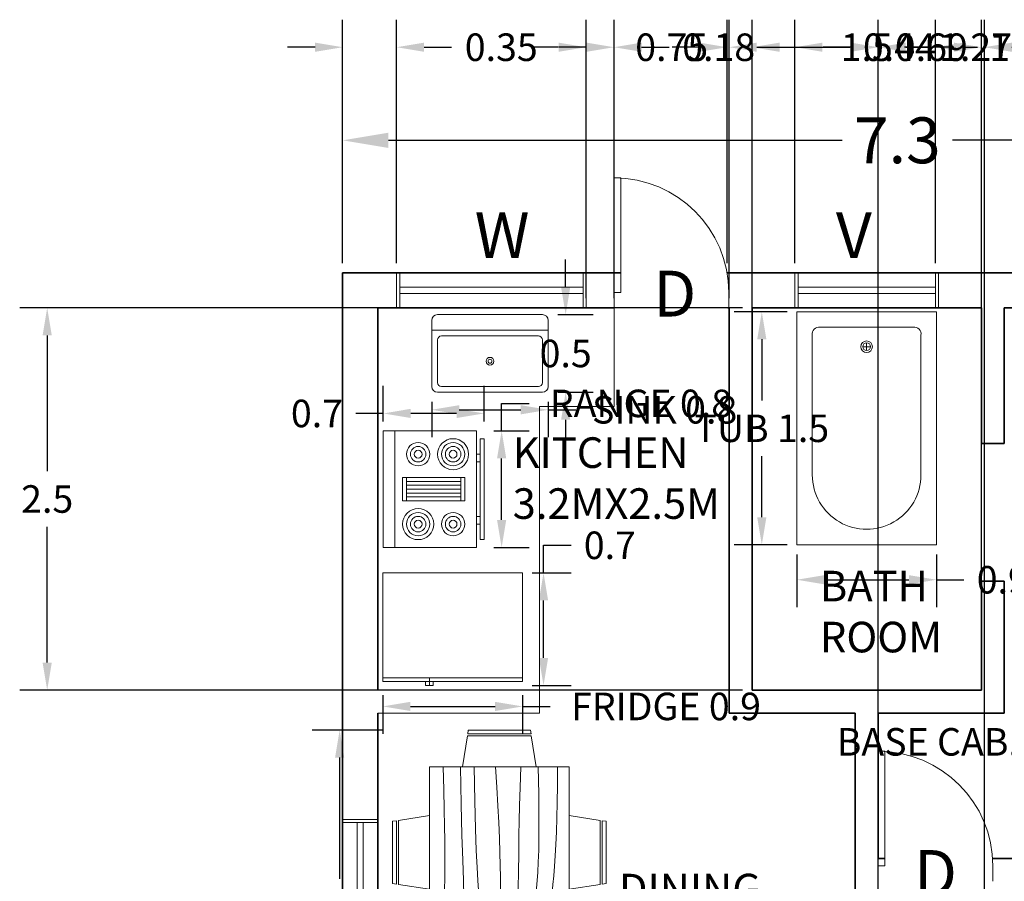
# Model space of a CAD drawing. Units: metres. Extents: x 40.9 to 56.1, y -1.4 to 24.2.
# Tile 6 of 7: x 43.1 to 49.6, y 18.6 to 24.2. Entities that reach past the tile are written whole.
import ezdxf

# ---------------------------------------------------------------- set-up
doc = ezdxf.new("R2010")
doc.units = ezdxf.units.M
doc.header["$MEASUREMENT"] = 0
for name, color, linetype, lineweight in [('A-ANNO-DIMS', 2, 'Continuous', 18), ('A-ANNO-TEXT', 7, 'Continuous', 18), ('A-AREA-IDEN', 7, 'Continuous', 18), ('A-DOOR', 3, 'Continuous', 18), ('A-EQPM', 8, 'Continuous', 18), ('A-FLOR-CASE', 9, 'Continuous', 18), ('A-FLOR-FIXT', 9, 'Continuous', 18), ('A-FURN', 8, 'Continuous', 18), ('A-GLAZ', 4, 'Continuous', 18), ('A-WALL', 7, 'Continuous', 35)]:
    doc.layers.add(name, color=color, linetype=linetype, lineweight=lineweight)
doc.styles.get("Standard").update_dxf_attribs({"font": 'arial.ttf'})
doc.dimstyles.get("Standard").update_dxf_attribs({"dimtxt": 0.18, "dimasz": 0.18, "dimexe": 0.18, "dimexo": 0.0625, "dimgap": 0.09, "dimtad": 0, "dimtih": 1, "dimtoh": 1, "dimdec": 1, "dimzin": 0, "dimdsep": 46, "dimtxsty": 'Standard', "dimcen": 0.09, "dimadec": 0, "dimazin": 0, "dimtfac": 1, "dimtdec": 1, "dimtofl": 0, "dimtmove": 0, "dimatfit": 3, "dimfxl": 1, "dimtolj": 1, "dimtzin": 0, "dimarcsym": 0})

# ---------------------------------------------------------------- blocks, each defined once
blk = doc.blocks.new('*U2')
for p, q in [((0, 0), (0, -100)), ((750, 0), (750, -100))]:
    blk.add_line(p, q)
blk.add_lwpolyline([(0, 0), (0, 750), (43.75, 750), (43.75, 0)], close=True)
blk.add_arc((0, 0), 750, 0, 90)
blk = doc.blocks.new('Bath Tub - 26 x 60 in.')
for p, q in [((9, -17), (9, -19)), ((8, -18), (10, -18))]:
    blk.add_line(p, q)
blk.add_lwpolyline([(0, -36), (0, 0), (60, 0), (60, -36)], close=True)
for points in [[(6, -4), (42, -4)], [(4, -30), (4, -6)], [(42, -32), (6, -32)]]:
    blk.add_lwpolyline(points)
for radius in [1.5, 1]:
    blk.add_circle((9, -18), radius)
for centre, radius, start, end in [((5.75, -5.75), 1.77, 81.8699, 188.1301), ((42, -18), 14, 270, 90), ((5.75, -30.25), 1.77, 171.8699, 278.1301)]:
    blk.add_arc(centre, radius, start, end)
blk = doc.blocks.new('Dining Set - 36 x 72 in.')
for p, q in [((-22.2343, 26.00059), (-23.4847, 17.99762)), ((-22.2304, 26), (-5.7608, 26)), ((-22, 27.5), (-22.1562, 26.50042)), ((-5.8416, 26.5), (-22.1534, 26.5)), ((-22, 27.5), (-6, 27.5)), ((-5.8437, 26.49966), (-6, 27.5)), ((-4.5152, 17.99762), (-5.7655, 25.99926)), ((5.7657, 26.00059), (4.5153, 17.99762)), ((5.7696, 26), (22.2392, 26)), ((6, 27.5), (5.8438, 26.50042)), ((22.1584, 26.5), (5.8466, 26.5)), ((6, 27.5), (22, 27.5)), ((22.1563, 26.49966), (22, 27.5)), ((23.4848, 17.99762), (22.2345, 25.99926)), ((36, 18), (-36, 18)), ((-36, 18), (-36, -18)), ((36, -18), (36, 18)), ((-45.5, 8), (-44.5004, 8.15617)), ((-45.5, 8), (-45.5, -8)), ((-44.5, -8.15843), (-44.5, 8.15338)), ((-44.0006, 8.23428), (-35.9976, 9.48474)), ((-44, 8.23041), (-44, -8.23915)), ((44.0006, 8.23428), (35.9976, 9.48474)), ((44, 8.23041), (44, -8.23915)), ((44.5, -8.15843), (44.5, 8.15338)), ((45.5, 8), (44.5005, 8.15617)), ((45.5, 8), (45.5, -8)), ((-44.4997, -8.15631), (-45.5, -8)), ((-35.9976, -9.48476), (-43.9993, -8.2345)), ((35.9976, -9.48476), (43.9993, -8.2345)), ((44.4997, -8.15631), (45.5, -8)), ((-36, -18), (36, -18)), ((-22.2343, -26.0006), (-23.4847, -17.99762)), ((-4.5152, -17.99762), (-5.7655, -25.99928)), ((5.7657, -26.0006), (4.5153, -17.99762)), ((23.4848, -17.99762), (22.2345, -25.99928)), ((-22.2304, -26), (-5.7608, -26)), ((-22, -27.5), (-22.1562, -26.50044)), ((-5.8416, -26.5), (-22.1534, -26.5)), ((-22, -27.5), (-6, -27.5)), ((-5.8437, -26.49967), (-6, -27.5)), ((5.7696, -26), (22.2392, -26)), ((6, -27.5), (5.8438, -26.50044)), ((22.1584, -26.5), (5.8466, -26.5)), ((6, -27.5), (22, -27.5)), ((22.1563, -26.49967), (22, -27.5))]:
    blk.add_line(p, q)
for points in [[(-36, 15), (-31.1772, 14.97754), (-26.8079, 14.91406), (-22.8538, 14.81543), (-19.276, 14.6875), (-16.0362, 14.53613), (-13.0957, 14.36718), (-10.4159, 14.18652), (-7.9583, 14), (-5.6904, 13.81315), (-3.6035, 13.63021), (-1.6954, 13.45508), (0.0365, 13.29166), (1.5945, 13.14388), (2.9811, 13.01562), (4.1988, 12.9108), (5.25, 12.83333), (6.1393, 12.78613), (6.8802, 12.76823), (7.4883, 12.77767), (7.9792, 12.8125), (8.3685, 12.87077), (8.6719, 12.95052), (8.9049, 13.0498), (9.0833, 13.16666), (9.2205, 13.29899), (9.3216, 13.44401), (9.3895, 13.59879), (9.4271, 13.76041), (9.4373, 13.92594), (9.4232, 14.09245), (9.3875, 14.257), (9.3333, 14.41666), (9.2638, 14.56917), (9.1836, 14.71484), (9.0975, 14.85465), (9.0104, 14.98958), (8.9272, 15.1206), (8.8529, 15.2487), (8.7922, 15.37483), (8.75, 15.5), (8.7305, 15.62467), (8.7344, 15.74739), (8.7617, 15.86621), (8.8125, 15.97916), (8.8867, 16.08431), (8.9844, 16.17968), (9.1055, 16.26334), (9.25, 16.33333), (9.4189, 16.38802), (9.6172, 16.42708), (9.8506, 16.45052), (10.125, 16.45833), (10.4463, 16.45052), (10.8203, 16.42708), (11.2529, 16.38802), (11.75, 16.33333), (12.3184, 16.26318), (12.9694, 16.17838), (13.7151, 16.07991), (14.5677, 15.96875), (15.5395, 15.84586), (16.6426, 15.71224), (17.8893, 15.56884), (19.2917, 15.41666), (20.859, 15.25667), (22.5879, 15.08984), (24.4721, 14.91715), (26.5052, 14.73958), (28.6809, 14.5581), (30.9929, 14.3737), (33.4347, 14.18733), (36, 14)], [(-36, 10), (-28.9766, 10.14274), (-23.1725, 10.20442), (-18.4241, 10.19775), (-14.5677, 10.13541), (-11.4399, 10.03011), (-8.877, 9.89453), (-6.7154, 9.74137), (-4.7917, 9.58333), (-2.9698, 9.43082), (-1.2246, 9.28515), (0.4415, 9.14534), (2.026, 9.01041), (3.5266, 8.87939), (4.9408, 8.7513), (6.266, 8.62516), (7.5, 8.5), (8.6411, 8.37549), (9.6914, 8.2539), (10.6538, 8.13818), (11.5312, 8.03125), (12.3267, 7.93603), (13.043, 7.85547), (13.6831, 7.79248), (14.25, 7.75), (14.7471, 7.7303), (15.1797, 7.73307), (15.5537, 7.75732), (15.875, 7.80208), (16.1494, 7.86637), (16.3828, 7.94922), (16.5811, 8.04964), (16.75, 8.16666), (16.8944, 8.29915), (17.0143, 8.44531), (17.1089, 8.60319), (17.1771, 8.77083), (17.218, 8.94629), (17.2305, 9.1276), (17.2137, 9.31282), (17.1667, 9.5), (17.0895, 9.6875), (16.987, 9.875), (16.8649, 10.0625), (16.7292, 10.25), (16.5856, 10.4375), (16.4401, 10.625), (16.2985, 10.8125), (16.1667, 11), (16.05, 11.18733), (15.9518, 11.3737), (15.8752, 11.5581), (15.8229, 11.73958), (15.798, 11.91715), (15.8034, 12.08984), (15.842, 12.25667), (15.9167, 12.41666), (16.0295, 12.56836), (16.1784, 12.70833), (16.3605, 12.83268), (16.5729, 12.9375), (16.8127, 13.01888), (17.0768, 13.07291), (17.3625, 13.0957), (17.6667, 13.08333), (17.9894, 13.03312), (18.3418, 12.94726), (18.7382, 12.82918), (19.1927, 12.68229), (19.7195, 12.51001), (20.3327, 12.31575), (21.0465, 12.10294), (21.875, 11.875), (22.8357, 11.63354), (23.959, 11.37304), (25.2786, 11.08618), (26.8282, 10.76562), (28.6414, 10.40405), (30.752, 9.99414), (33.1936, 9.52856), (36, 9)], [(-36, 5.5), (-30.7157, 5.3348), (-26.069, 5.20963), (-21.9946, 5.11767), (-18.4271, 5.05208), (-15.3009, 5.00602), (-12.5508, 4.97265), (-10.1112, 4.94515), (-7.9167, 4.91666), (-5.909, 4.88167), (-4.0586, 4.83984), (-2.3429, 4.79215), (-0.7396, 4.73958), (0.7739, 4.6831), (2.22, 4.6237), (3.6213, 4.56233), (5, 4.5), (6.373, 4.43782), (7.7344, 4.3776), (9.0723, 4.32129), (10.375, 4.27083), (11.6309, 4.22819), (12.8281, 4.19531), (13.9551, 4.17415), (15, 4.16666), (15.954, 4.17448), (16.819, 4.19791), (17.6001, 4.23698), (18.3021, 4.29166), (18.9299, 4.36198), (19.4883, 4.44791), (19.9823, 4.54948), (20.4167, 4.66666), (20.7969, 4.79899), (21.1302, 4.94401), (21.4245, 5.09879), (21.6875, 5.26041), (21.9271, 5.42594), (22.1511, 5.59245), (22.3672, 5.757), (22.5834, 5.91666), (22.8065, 6.06868), (23.0404, 6.21093), (23.2879, 6.34147), (23.5521, 6.45833), (23.8358, 6.55957), (24.142, 6.64323), (24.4735, 6.70735), (24.8334, 6.75), (25.2235, 6.76969), (25.642, 6.76692), (26.0858, 6.74267), (26.5521, 6.69791), (27.0379, 6.63362), (27.5404, 6.55078), (28.0565, 6.45036), (28.5834, 6.33333), (29.1242, 6.19987), (29.7071, 6.04687), (30.3661, 5.87044), (31.1354, 5.66666), (32.0493, 5.43164), (33.142, 5.16146), (34.4475, 4.85221), (36, 4.5)], [(-36, -1), (-30.7915, -0.6591), (-26.0195, -0.38216), (-21.6519, -0.16284), (-17.6563, 0.00521), (-14.0005, 0.12833), (-10.6523, 0.21289), (-7.5796, 0.26522), (-4.75, 0.29166), (-2.134, 0.29793), (0.2878, 0.28711), (2.5317, 0.26163), (4.6146, 0.22396), (6.5529, 0.17651), (8.3633, 0.12174), (10.0623, 0.06209), (11.6667, 0), (13.1899, -0.06201), (14.6341, -0.1211), (15.9982, -0.17432), (17.2813, -0.21875), (18.4823, -0.25147), (19.6003, -0.26953), (20.6343, -0.27002), (21.5834, -0.25), (22.4481, -0.20768), (23.2357, -0.14584), (23.9549, -0.06836), (24.6146, 0.02083), (25.2235, 0.11784), (25.7904, 0.21875), (26.3241, 0.31966), (26.8334, 0.41666), (27.3265, 0.50618), (27.8099, 0.58593), (28.2894, 0.65397), (28.7709, 0.70833), (29.2601, 0.74707), (29.763, 0.76823), (30.2855, 0.76985), (30.8334, 0.75), (31.4088, 0.70784), (31.9994, 0.64713), (32.589, 0.57275), (33.1615, 0.48958), (33.7008, 0.4025), (34.1908, 0.3164), (34.6153, 0.23616), (34.9584, 0.16666), (35.2099, 0.11165), (35.3848, 0.07031), (35.504, 0.04069), (35.5886, 0.02083), (35.6594, 0.00879), (35.7377, 0.0026), (35.8442, 0.00032), (36, 0)], [(-36, -6.5), (-27.1843, -6.31267), (-20.084, -6.1263), (-14.469, -5.9419), (-10.1094, -5.76042), (-6.7752, -5.58285), (-4.2363, -5.41016), (-2.2629, -5.24333), (-0.625, -5.08334), (0.8708, -4.93099), (2.2715, -4.78646), (3.5872, -4.64974), (4.8281, -4.52084), (6.0046, -4.39974), (7.127, -4.28646), (8.2053, -4.18099), (9.25, -4.08334), (10.2705, -3.99382), (11.2734, -3.91407), (12.2647, -3.84603), (13.25, -3.79167), (14.2354, -3.75293), (15.2266, -3.73177), (16.2295, -3.73015), (17.25, -3.75), (18.2912, -3.79248), (19.3451, -3.85547), (20.4009, -3.93604), (21.4479, -4.03125), (22.4754, -4.13819), (23.4727, -4.25391), (24.4289, -4.37549), (25.3334, -4.5), (26.1785, -4.62492), (26.9694, -4.74935), (27.7145, -4.87281), (28.4219, -4.99479), (29.1, -5.11483), (29.7572, -5.23242), (30.4016, -5.34709), (31.0417, -5.45834), (31.6837, -5.56437), (32.3262, -5.65821), (32.9658, -5.73153), (33.599, -5.77604), (34.2224, -5.78345), (34.8327, -5.74545), (35.4264, -5.65373), (36, -5.5)], [(-36, -10), (-26.4022, -9.81299), (-18.4675, -9.62891), (-11.9839, -9.45069), (-6.7396, -9.28125), (-2.5226, -9.12354), (0.8789, -8.98047), (3.6769, -8.85498), (6.0833, -8.75), (8.2767, -8.66765), (10.3021, -8.60677), (12.1712, -8.56543), (13.8958, -8.54167), (15.4876, -8.53353), (16.9583, -8.53907), (18.3197, -8.55632), (19.5834, -8.58334), (20.7616, -8.61841), (21.8685, -8.66081), (22.9188, -8.71004), (23.9271, -8.76563), (24.9081, -8.82707), (25.8763, -8.89388), (26.8465, -8.96558), (27.8334, -9.04167), (28.8474, -9.12118), (29.8828, -9.20117), (30.93, -9.27824), (31.9792, -9.34896), (33.0205, -9.40991), (34.0443, -9.45768), (35.0407, -9.48885), (36, -9.5)], [(-36, -14.5), (-30.0881, -14.33513), (-25.0332, -14.21224), (-20.7312, -14.12647), (-17.0781, -14.07292), (-13.97, -14.04671), (-11.3027, -14.04297), (-8.9724, -14.05681), (-6.875, -14.08334), (-4.9224, -14.11833), (-3.0905, -14.16016), (-1.3709, -14.20785), (0.2448, -14.26042), (1.7647, -14.3169), (3.1973, -14.3763), (4.5507, -14.43767), (5.8333, -14.5), (7.0554, -14.5621), (8.235, -14.62175), (9.3922, -14.67652), (10.5469, -14.72396), (11.7192, -14.76164), (12.929, -14.78711), (14.1965, -14.79794), (15.5417, -14.79167), (16.9933, -14.76424), (18.6152, -14.70508), (20.4804, -14.60197), (22.6615, -14.44271), (25.2312, -14.21509), (28.2624, -13.9069), (31.8277, -13.50594), (36, -13)]]:
    blk.add_lwpolyline(points)
blk = doc.blocks.new('Refrigerator-2 door - 36 in top')
for p, q in [((0, -26.999999), (36, -26.999999)), ((12, -26.999999), (12, -28.999999)), ((11, -27.999999), (11, -28.999999)), ((11, -28.999999), (13, -28.999999)), ((13, -28.999999), (13, -27.999999))]:
    blk.add_line(p, q)
blk.add_lwpolyline([(0, -27.999999), (0, 0), (36, 0), (36, -27.999999)], close=True)
blk = doc.blocks.new('Range-Oven - 30 in top')
for p, q in [((0, -3), (30, -3)), ((12, -6), (18, -6)), ((13, -20), (13, -6)), ((14, -6), (14, -20)), ((15, -20), (15, -6)), ((16, -6), (16, -20)), ((17, -20), (17, -6)), ((18, -20), (12, -20)), ((6, -24), (6, -25)), ((8, -25), (8, -24)), ((22, -25), (22, -24)), ((24, -24), (24, -25))]:
    blk.add_line(p, q)
for points in [[(0, -24), (0, 0), (30, 0), (30, -24)], [(12, -21), (12, -5), (18, -5), (18, -21)], [(2, -26), (2, -25), (28, -25), (28, -26)]]:
    blk.add_lwpolyline(points, close=True)
for centre, radius in [((6, -9), 4), ((6, -9), 3), ((6, -9), 2), ((24, -9), 3), ((24, -9), 2), ((6, -9), 1), ((24, -9), 1), ((6, -18), 3), ((24, -18), 4), ((24, -18), 3), ((6, -18), 2), ((6, -18), 1), ((24, -18), 2), ((24, -18), 1)]:
    blk.add_circle(centre, radius)
blk = doc.blocks.new('Sink-single - 30 in top')
blk.add_line((-15, -3.999996), (15, -3.999996))
for points in [[(-13.5, 0), (13.5, 0)], [(-15, -18.499996), (-15, -1.5)], [(15, -1.5), (15, -18.499996)], [(-13.5, -17.499996), (-13.5, -6.499996)], [(-12.5, -5.499996), (12.5, -5.499996)], [(13.5, -6.499996), (13.5, -17.499996)], [(13.5, -19.999996), (-13.5, -19.999996)], [(12.5, -18.499996), (-12.5, -18.499996)]]:
    blk.add_lwpolyline(points)
for radius in [1, 0.5]:
    blk.add_circle((0, -11.999996), radius)
for centre, radius, start, end in [((-13.5, -1.5), 1.5, 90, 180), ((13.5, -1.5), 1.5, 0, 90), ((-12.5, -6.499996), 1, 90, 180), ((12.5, -6.499996), 1, 0, 90), ((-12.5, -17.499996), 1, 180, 270), ((12.5, -17.499996), 1, 270, 0), ((-13.5, -18.499996), 1.5, 180, 270), ((13.5, -18.499996), 1.5, 270, 0)]:
    blk.add_arc(centre, radius, start, end)
blk = doc.blocks.new('*D45')
at = {"layer": 'A-ANNO-DIMS', "color": 0, "lineweight": -2, "transparency": 16777216}
for p, q in [((45.2552, 22.6498), (45.2552, 23.6329)), ((52.5152, 22.6498), (52.5152, 23.6329)), ((45.5552, 23.4529), (48.5233, 23.4529)), ((52.2152, 23.4529), (49.2471, 23.4529))]:
    blk.add_line(p, q, dxfattribs=at)
at = {"layer": 'A-ANNO-DIMS', "color": 0, "transparency": 16777216}
for points in [[(45.5552, 23.5029), (45.5552, 23.4029), (45.2552, 23.4529)], [(52.2152, 23.5029), (52.2152, 23.4029), (52.5152, 23.4529)]]:
    blk.add_solid(points, dxfattribs=at)
at = {"layer": 'Defpoints', "color": 0, "transparency": 16777216}
for p in [(52.5152, 23.4529), (45.2552, 22.5873), (52.5152, 22.5873)]:
    blk.add_point(p, dxfattribs=at)
at = {"layer": 'A-ANNO-DIMS', "color": 0, "transparency": 16777216, "insert": (48.8852, 23.4529), "char_height": 0.3, "attachment_point": 5}
blk.add_mtext('\\A1;7.3', dxfattribs=at)
blk = doc.blocks.new('WIN-1200-PLAN')
for p, q in [((-0.0002, 0.0003), (-0.0002, 0.2303)), ((0.0198, 0.0003), (0.0198, 0.2303)), ((1.2198, 0.0003), (1.2198, 0.2303)), ((1.2398, 0.0003), (1.2398, 0.2303)), ((0.0198, 0.1353), (1.2198, 0.1353)), ((0.0198, 0.0953), (1.2198, 0.0953))]:
    blk.add_line(p, q)
blk = doc.blocks.new('VENT-900-PLAN')
for p, q in [((0.0002, 0.0003), (0.0002, 0.2303)), ((0.0202, 0.0003), (0.0202, 0.2303)), ((0.9202, 0.0003), (0.9202, 0.2303)), ((0.9402, 0.0003), (0.9402, 0.2303)), ((0.0202, 0.1353), (0.9202, 0.1353)), ((0.0202, 0.0953), (0.9202, 0.0953))]:
    blk.add_line(p, q)
blk = doc.blocks.new('*D93')
at = {"layer": 'A-ANNO-DIMS', "color": 0, "lineweight": -2, "transparency": 16777216}
for p, q in [((48.1645, 22.3318), (47.8184, 22.3318)), ((47.9984, 22.1518), (47.9984, 21.7517)), ((47.9984, 20.9878), (47.9984, 21.3879)), ((48.1645, 20.8078), (47.8184, 20.8078))]:
    blk.add_line(p, q, dxfattribs=at)
at = {"layer": 'A-ANNO-DIMS', "color": 0, "transparency": 16777216}
for points in [[(47.9684, 22.1518), (48.0284, 22.1518), (47.9984, 22.3318)], [(47.9684, 20.9878), (48.0284, 20.9878), (47.9984, 20.8078)]]:
    blk.add_solid(points, dxfattribs=at)
at = {"layer": 'Defpoints', "color": 0, "transparency": 16777216}
for p in [(48.227, 22.3318), (47.9984, 20.8078), (48.227, 20.8078)]:
    blk.add_point(p, dxfattribs=at)
at = {"layer": 'A-ANNO-DIMS', "color": 0, "transparency": 16777216, "insert": (47.9984, 21.5698), "char_height": 0.18, "attachment_point": 5}
blk.add_mtext('\\A1;TUB 1.5', dxfattribs=at)
blk = doc.blocks.new('*D94')
at = {"layer": 'A-ANNO-DIMS', "color": 0, "lineweight": -2, "transparency": 16777216}
for p, q in [((48.227, 20.7453), (48.227, 20.3992)), ((49.1414, 20.7453), (49.1414, 20.3992)), ((48.407, 20.5792), (48.9614, 20.5792)), ((49.1414, 20.5792), (49.3214, 20.5792))]:
    blk.add_line(p, q, dxfattribs=at)
at = {"layer": 'A-ANNO-DIMS', "color": 0, "transparency": 16777216}
for points in [[(48.407, 20.6092), (48.407, 20.5492), (48.227, 20.5792)], [(48.9614, 20.6092), (48.9614, 20.5492), (49.1414, 20.5792)]]:
    blk.add_solid(points, dxfattribs=at)
at = {"layer": 'Defpoints', "color": 0, "transparency": 16777216}
for p in [(48.227, 20.8078), (49.1414, 20.8078), (49.1414, 20.5792)]:
    blk.add_point(p, dxfattribs=at)
at = {"layer": 'A-ANNO-DIMS', "color": 0, "transparency": 16777216, "insert": (49.5754, 20.5792), "char_height": 0.18, "attachment_point": 5}
blk.add_mtext('\\A1;0.9', dxfattribs=at)
blk = doc.blocks.new('*D97')
at = {"layer": 'A-ANNO-DIMS', "color": 0, "lineweight": -2, "transparency": 16777216}
for p, q in [((45.52, 19.5966), (45.0558, 19.5966)), ((45.2358, 19.4166), (45.2358, 18.624)), ((45.2358, 17.4652), (45.2358, 18.2578)), ((45.52, 17.2852), (45.0558, 17.2852))]:
    blk.add_line(p, q, dxfattribs=at)
at = {"layer": 'A-ANNO-DIMS', "color": 0, "transparency": 16777216}
for points in [[(45.2058, 19.4166), (45.2658, 19.4166), (45.2358, 19.5966)], [(45.2058, 17.4652), (45.2658, 17.4652), (45.2358, 17.2852)]]:
    blk.add_solid(points, dxfattribs=at)
at = {"layer": 'Defpoints', "color": 0, "transparency": 16777216}
for p in [(45.5825, 19.5966), (45.2358, 17.2852), (45.5825, 17.2852)]:
    blk.add_point(p, dxfattribs=at)
at = {"layer": 'A-ANNO-DIMS', "color": 0, "transparency": 16777216, "insert": (45.2358, 18.4409), "char_height": 0.18, "attachment_point": 5}
blk.add_mtext('\\A1;DINING SET 2.3', dxfattribs=at)
blk = doc.blocks.new('*D105')
at = {"layer": 'A-ANNO-DIMS', "color": 0, "lineweight": -2, "transparency": 16777216}
for p, q in [((45.5186, 19.8254), (45.5186, 19.5708)), ((46.433, 19.8254), (46.433, 19.5708)), ((45.6986, 19.7508), (46.253, 19.7508)), ((46.433, 19.7508), (46.613, 19.7508))]:
    blk.add_line(p, q, dxfattribs=at)
at = {"layer": 'A-ANNO-DIMS', "color": 0, "transparency": 16777216}
for points in [[(45.6986, 19.7808), (45.6986, 19.7208), (45.5186, 19.7508)], [(46.253, 19.7808), (46.253, 19.7208), (46.433, 19.7508)]]:
    blk.add_solid(points, dxfattribs=at)
at = {"layer": 'Defpoints', "color": 0, "transparency": 16777216}
for p in [(45.5186, 19.8879), (46.433, 19.8879), (46.433, 19.7508)]:
    blk.add_point(p, dxfattribs=at)
at = {"layer": 'A-ANNO-DIMS', "color": 0, "transparency": 16777216, "insert": (47.3718, 19.7508), "char_height": 0.18, "attachment_point": 5}
blk.add_mtext('\\A1;FRIDGE 0.9', dxfattribs=at)
blk = doc.blocks.new('*D106')
at = {"layer": 'A-ANNO-DIMS', "color": 0, "lineweight": -2, "transparency": 16777216}
for p, q in [((46.5701, 20.6245), (46.5701, 20.8045)), ((46.5701, 20.8045), (46.7501, 20.8045)), ((46.4955, 20.6245), (46.7501, 20.6245)), ((46.5701, 20.0679), (46.5701, 20.4445)), ((46.4955, 19.8879), (46.7501, 19.8879))]:
    blk.add_line(p, q, dxfattribs=at)
at = {"layer": 'A-ANNO-DIMS', "color": 0, "transparency": 16777216}
for points in [[(46.5401, 20.4445), (46.6001, 20.4445), (46.5701, 20.6245)], [(46.5401, 20.0679), (46.6001, 20.0679), (46.5701, 19.8879)]]:
    blk.add_solid(points, dxfattribs=at)
at = {"layer": 'Defpoints', "color": 0, "transparency": 16777216}
for p in [(46.433, 20.6245), (46.5701, 20.6245), (46.433, 19.8879)]:
    blk.add_point(p, dxfattribs=at)
at = {"layer": 'A-ANNO-DIMS', "color": 0, "transparency": 16777216, "insert": (47.004, 20.8045), "char_height": 0.18, "attachment_point": 5}
blk.add_mtext('\\A1;0.7', dxfattribs=at)
blk = doc.blocks.new('*D107')
at = {"layer": 'A-ANNO-DIMS', "color": 0, "lineweight": -2, "transparency": 16777216}
for p, q in [((46.2958, 21.5526), (46.2958, 21.7326)), ((46.2958, 21.7326), (46.4758, 21.7326)), ((46.244, 21.5526), (46.4758, 21.5526)), ((46.2958, 20.9706), (46.2958, 21.3726)), ((46.244, 20.7906), (46.4758, 20.7906))]:
    blk.add_line(p, q, dxfattribs=at)
at = {"layer": 'A-ANNO-DIMS', "color": 0, "transparency": 16777216}
for points in [[(46.2658, 21.3726), (46.3258, 21.3726), (46.2958, 21.5526)], [(46.2658, 20.9706), (46.3258, 20.9706), (46.2958, 20.7906)]]:
    blk.add_solid(points, dxfattribs=at)
at = {"layer": 'Defpoints', "color": 0, "transparency": 16777216}
for p in [(46.1815, 21.5526), (46.2958, 21.5526), (46.1815, 20.7906)]:
    blk.add_point(p, dxfattribs=at)
at = {"layer": 'A-ANNO-DIMS', "color": 0, "transparency": 16777216, "insert": (47.2072, 21.7326), "char_height": 0.18, "attachment_point": 5}
blk.add_mtext('\\A1;RANGE 0.8', dxfattribs=at)
blk = doc.blocks.new('*D108')
at = {"layer": 'A-ANNO-DIMS', "color": 0, "lineweight": -2, "transparency": 16777216}
for p, q in [((45.5211, 21.6151), (45.5211, 21.8469)), ((46.1815, 21.6151), (46.1815, 21.8469)), ((45.5211, 21.6669), (45.3411, 21.6669)), ((46.0015, 21.6669), (45.7011, 21.6669))]:
    blk.add_line(p, q, dxfattribs=at)
at = {"layer": 'A-ANNO-DIMS', "color": 0, "transparency": 16777216}
for points in [[(45.7011, 21.6969), (45.7011, 21.6369), (45.5211, 21.6669)], [(46.0015, 21.6969), (46.0015, 21.6369), (46.1815, 21.6669)]]:
    blk.add_solid(points, dxfattribs=at)
at = {"layer": 'Defpoints', "color": 0, "transparency": 16777216}
for p in [(45.5211, 21.6669), (45.5211, 21.5526), (46.1815, 21.5526)]:
    blk.add_point(p, dxfattribs=at)
at = {"layer": 'A-ANNO-DIMS', "color": 0, "transparency": 16777216, "insert": (45.0873, 21.6669), "char_height": 0.18, "attachment_point": 5}
blk.add_mtext('\\A1;0.7', dxfattribs=at)
blk = doc.blocks.new('*D109')
at = {"layer": 'A-ANNO-DIMS', "color": 0, "lineweight": -2, "transparency": 16777216}
for p, q in [((45.8385, 21.7426), (45.8385, 21.5108)), ((46.6005, 21.7426), (46.6005, 21.5108)), ((46.0185, 21.6908), (46.4205, 21.6908)), ((46.6005, 21.6908), (46.7805, 21.6908))]:
    blk.add_line(p, q, dxfattribs=at)
at = {"layer": 'A-ANNO-DIMS', "color": 0, "transparency": 16777216}
for points in [[(46.0185, 21.7208), (46.0185, 21.6608), (45.8385, 21.6908)], [(46.4205, 21.7208), (46.4205, 21.6608), (46.6005, 21.6908)]]:
    blk.add_solid(points, dxfattribs=at)
at = {"layer": 'Defpoints', "color": 0, "transparency": 16777216}
for p in [(45.8385, 21.8051), (46.6005, 21.8051), (46.6005, 21.6908)]:
    blk.add_point(p, dxfattribs=at)
at = {"layer": 'A-ANNO-DIMS', "color": 0, "transparency": 16777216, "insert": (47.3625, 21.6908), "char_height": 0.18, "attachment_point": 5}
blk.add_mtext('\\A1;SINK 0.8', dxfattribs=at)
blk = doc.blocks.new('*D110')
at = {"layer": 'A-ANNO-DIMS', "color": 0, "lineweight": -2, "transparency": 16777216}
for p, q in [((46.7148, 22.4931), (46.7148, 22.6731)), ((46.663, 22.3131), (46.8948, 22.3131)), ((46.663, 21.8051), (46.8948, 21.8051)), ((46.7148, 21.6251), (46.7148, 21.4451))]:
    blk.add_line(p, q, dxfattribs=at)
at = {"layer": 'A-ANNO-DIMS', "color": 0, "transparency": 16777216}
for points in [[(46.6848, 22.4931), (46.7448, 22.4931), (46.7148, 22.3131)], [(46.6848, 21.6251), (46.7448, 21.6251), (46.7148, 21.8051)]]:
    blk.add_solid(points, dxfattribs=at)
at = {"layer": 'Defpoints', "color": 0, "transparency": 16777216}
for p in [(46.6005, 22.3131), (46.7148, 22.3131), (46.6005, 21.8051)]:
    blk.add_point(p, dxfattribs=at)
at = {"layer": 'A-ANNO-DIMS', "color": 0, "transparency": 16777216, "insert": (46.7148, 22.0591), "char_height": 0.18, "attachment_point": 5}
blk.add_mtext('\\A1;0.5', dxfattribs=at)
blk = doc.blocks.new('*D111')
at = {"layer": 'A-ANNO-DIMS', "color": 0, "lineweight": -2, "transparency": 16777216}
for p, q in [((50.4115, 19.4502), (50.4115, 19.6992)), ((51.2878, 19.4502), (51.2878, 19.6992)), ((50.4115, 19.5192), (50.2315, 19.5192)), ((51.1078, 19.5192), (50.5915, 19.5192))]:
    blk.add_line(p, q, dxfattribs=at)
at = {"layer": 'A-ANNO-DIMS', "color": 0, "transparency": 16777216}
for points in [[(50.5915, 19.5492), (50.5915, 19.4892), (50.4115, 19.5192)], [(51.1078, 19.5492), (51.1078, 19.4892), (51.2878, 19.5192)]]:
    blk.add_solid(points, dxfattribs=at)
at = {"layer": 'Defpoints', "color": 0, "transparency": 16777216}
for p in [(50.4115, 19.5192), (50.4115, 19.3877), (51.2878, 19.3877)]:
    blk.add_point(p, dxfattribs=at)
at = {"layer": 'A-ANNO-DIMS', "color": 0, "transparency": 16777216, "insert": (49.2827, 19.5192), "char_height": 0.18, "attachment_point": 5}
blk.add_mtext('\\A1;BASE CAB. 0.9', dxfattribs=at)
blk = doc.blocks.new('*D132')
at = {"layer": 'A-ANNO-DIMS', "color": 0, "lineweight": -2, "transparency": 16777216}
for p, q in [((47.9352, 19.9198), (47.9352, 24.2418)), ((49.4352, 19.9198), (49.4352, 24.2418)), ((48.1152, 24.0618), (48.4391, 24.0618)), ((49.2552, 24.0618), (48.9313, 24.0618))]:
    blk.add_line(p, q, dxfattribs=at)
at = {"layer": 'A-ANNO-DIMS', "color": 0, "transparency": 16777216}
for points in [[(48.1152, 24.0918), (48.1152, 24.0318), (47.9352, 24.0618)], [(49.2552, 24.0918), (49.2552, 24.0318), (49.4352, 24.0618)]]:
    blk.add_solid(points, dxfattribs=at)
at = {"layer": 'Defpoints', "color": 0, "transparency": 16777216}
for p in [(49.4352, 24.0618), (47.9352, 19.8573), (49.4352, 19.8573)]:
    blk.add_point(p, dxfattribs=at)
at = {"layer": 'A-ANNO-DIMS', "color": 0, "transparency": 16777216, "insert": (48.6852, 24.0618), "char_height": 0.18, "attachment_point": 5}
blk.add_mtext('\\A1;1.5', dxfattribs=at)
blk = doc.blocks.new('*D133')
at = {"layer": 'A-ANNO-DIMS', "color": 0, "lineweight": -2, "transparency": 16777216}
for p, q in [((47.8727, 22.3573), (43.1421, 22.3573)), ((43.3221, 22.1773), (43.3221, 21.2892)), ((43.3221, 20.0373), (43.3221, 20.9253)), ((47.8727, 19.8573), (43.1421, 19.8573))]:
    blk.add_line(p, q, dxfattribs=at)
at = {"layer": 'A-ANNO-DIMS', "color": 0, "transparency": 16777216}
for points in [[(43.2921, 22.1773), (43.3521, 22.1773), (43.3221, 22.3573)], [(43.2921, 20.0373), (43.3521, 20.0373), (43.3221, 19.8573)]]:
    blk.add_solid(points, dxfattribs=at)
at = {"layer": 'Defpoints', "color": 0, "transparency": 16777216}
for p in [(43.3221, 22.3573), (47.9352, 22.3573), (47.9352, 19.8573)]:
    blk.add_point(p, dxfattribs=at)
at = {"layer": 'A-ANNO-DIMS', "color": 0, "transparency": 16777216, "insert": (43.3221, 21.1073), "char_height": 0.18, "attachment_point": 5}
blk.add_mtext('\\A1;2.5', dxfattribs=at)
blk = doc.blocks.new('*D136')
at = {"layer": 'A-ANNO-DIMS', "color": 0, "lineweight": -2, "transparency": 16777216}
for p, q in [((48.7602, 14.8764), (48.7602, 24.2418)), ((49.4546, 14.8764), (49.4546, 24.2418)), ((48.5802, 24.0618), (48.4002, 24.0618)), ((49.6346, 24.0618), (49.8146, 24.0618))]:
    blk.add_line(p, q, dxfattribs=at)
at = {"layer": 'A-ANNO-DIMS', "color": 0, "transparency": 16777216}
for points in [[(48.5802, 24.0918), (48.5802, 24.0318), (48.7602, 24.0618)], [(49.6346, 24.0918), (49.6346, 24.0318), (49.4546, 24.0618)]]:
    blk.add_solid(points, dxfattribs=at)
at = {"layer": 'Defpoints', "color": 0, "transparency": 16777216}
for p in [(49.4546, 24.0618), (48.7602, 14.8139), (49.4546, 14.8139)]:
    blk.add_point(p, dxfattribs=at)
at = {"layer": 'A-ANNO-DIMS', "color": 0, "transparency": 16777216, "insert": (49.1074, 24.0618), "char_height": 0.18, "attachment_point": 5}
blk.add_mtext('\\A1;0.69', dxfattribs=at)
blk = doc.blocks.new('*D143')
at = {"layer": 'A-ANNO-DIMS', "color": 0, "lineweight": -2, "transparency": 16777216}
for p, q in [((45.2552, 22.6498), (45.2552, 24.2418)), ((45.6088, 22.6498), (45.6088, 24.2418)), ((45.0752, 24.0618), (44.8952, 24.0618)), ((45.7888, 24.0618), (45.9688, 24.0618))]:
    blk.add_line(p, q, dxfattribs=at)
at = {"layer": 'A-ANNO-DIMS', "color": 0, "transparency": 16777216}
for points in [[(45.0752, 24.0918), (45.0752, 24.0318), (45.2552, 24.0618)], [(45.7888, 24.0918), (45.7888, 24.0318), (45.6088, 24.0618)]]:
    blk.add_solid(points, dxfattribs=at)
at = {"layer": 'Defpoints', "color": 0, "transparency": 16777216}
for p in [(45.6088, 24.0618), (45.2552, 22.5873), (45.6088, 22.5873)]:
    blk.add_point(p, dxfattribs=at)
at = {"layer": 'A-ANNO-DIMS', "color": 0, "transparency": 16777216, "insert": (46.2933, 24.0618), "char_height": 0.18, "attachment_point": 5}
blk.add_mtext('\\A1;0.35', dxfattribs=at)
blk = doc.blocks.new('*D144')
at = {"layer": 'A-ANNO-DIMS', "color": 0, "lineweight": -2, "transparency": 16777216}
for p, q in [((46.8488, 22.4198), (46.8488, 24.2418)), ((47.032, 22.4198), (47.032, 24.2418)), ((46.6688, 24.0618), (46.4888, 24.0618)), ((47.212, 24.0618), (47.392, 24.0618))]:
    blk.add_line(p, q, dxfattribs=at)
at = {"layer": 'A-ANNO-DIMS', "color": 0, "transparency": 16777216}
for points in [[(46.6688, 24.0918), (46.6688, 24.0318), (46.8488, 24.0618)], [(47.212, 24.0918), (47.212, 24.0318), (47.032, 24.0618)]]:
    blk.add_solid(points, dxfattribs=at)
at = {"layer": 'Defpoints', "color": 0, "transparency": 16777216}
for p in [(47.032, 24.0618), (46.8488, 22.3573), (47.032, 22.3573)]:
    blk.add_point(p, dxfattribs=at)
at = {"layer": 'A-ANNO-DIMS', "color": 0, "transparency": 16777216, "insert": (47.716, 24.0618), "char_height": 0.18, "attachment_point": 5}
blk.add_mtext('\\A1;0.18', dxfattribs=at)
blk = doc.blocks.new('*D145')
at = {"layer": 'A-ANNO-DIMS', "color": 0, "lineweight": -2, "transparency": 16777216}
for p, q in [((47.032, 22.4198), (47.032, 24.2418)), ((47.7852, 22.4198), (47.7852, 24.2418)), ((46.852, 24.0618), (46.672, 24.0618)), ((47.9652, 24.0618), (48.1452, 24.0618))]:
    blk.add_line(p, q, dxfattribs=at)
at = {"layer": 'A-ANNO-DIMS', "color": 0, "transparency": 16777216}
for points in [[(46.852, 24.0918), (46.852, 24.0318), (47.032, 24.0618)], [(47.9652, 24.0918), (47.9652, 24.0318), (47.7852, 24.0618)]]:
    blk.add_solid(points, dxfattribs=at)
at = {"layer": 'Defpoints', "color": 0, "transparency": 16777216}
for p in [(47.7852, 24.0618), (47.032, 22.3573), (47.7852, 22.3573)]:
    blk.add_point(p, dxfattribs=at)
at = {"layer": 'A-ANNO-DIMS', "color": 0, "transparency": 16777216, "insert": (47.4086, 24.0618), "char_height": 0.18, "attachment_point": 5}
blk.add_mtext('\\A1;0.75', dxfattribs=at)
blk = doc.blocks.new('*D146')
at = {"layer": 'A-ANNO-DIMS', "color": 0, "lineweight": -2, "transparency": 16777216}
for p, q in [((47.7707, 22.6498), (47.7707, 24.2418)), ((48.2152, 22.6498), (48.2152, 24.2418)), ((47.5907, 24.0618), (47.4107, 24.0618)), ((48.3952, 24.0618), (48.5752, 24.0618))]:
    blk.add_line(p, q, dxfattribs=at)
at = {"layer": 'A-ANNO-DIMS', "color": 0, "transparency": 16777216}
for points in [[(47.5907, 24.0918), (47.5907, 24.0318), (47.7707, 24.0618)], [(48.3952, 24.0918), (48.3952, 24.0318), (48.2152, 24.0618)]]:
    blk.add_solid(points, dxfattribs=at)
at = {"layer": 'Defpoints', "color": 0, "transparency": 16777216}
for p in [(48.2152, 24.0618), (47.7707, 22.5873), (48.2152, 22.5873)]:
    blk.add_point(p, dxfattribs=at)
at = {"layer": 'A-ANNO-DIMS', "color": 0, "transparency": 16777216, "insert": (48.8986, 24.0618), "char_height": 0.18, "attachment_point": 5}
blk.add_mtext('\\A1;0.44', dxfattribs=at)
blk = doc.blocks.new('*D147')
at = {"layer": 'A-ANNO-DIMS', "color": 0, "lineweight": -2, "transparency": 16777216}
for p, q in [((49.1352, 22.6498), (49.1352, 24.2418)), ((50.3152, 22.6498), (50.3152, 24.2418)), ((49.3152, 24.0618), (49.4097, 24.0618)), ((50.1352, 24.0618), (50.0407, 24.0618))]:
    blk.add_line(p, q, dxfattribs=at)
at = {"layer": 'A-ANNO-DIMS', "color": 0, "transparency": 16777216}
for points in [[(49.3152, 24.0918), (49.3152, 24.0318), (49.1352, 24.0618)], [(50.1352, 24.0918), (50.1352, 24.0318), (50.3152, 24.0618)]]:
    blk.add_solid(points, dxfattribs=at)
at = {"layer": 'Defpoints', "color": 0, "transparency": 16777216}
for p in [(50.3152, 24.0618), (49.1352, 22.5873), (50.3152, 22.5873)]:
    blk.add_point(p, dxfattribs=at)
at = {"layer": 'A-ANNO-DIMS', "color": 0, "transparency": 16777216, "insert": (49.7252, 24.0618), "char_height": 0.18, "attachment_point": 5}
blk.add_mtext('\\A1;1.18', dxfattribs=at)
blk = doc.blocks.new('*D154')
at = {"layer": 'A-ANNO-DIMS', "color": 0, "lineweight": -2, "transparency": 16777216}
for p, q in [((48.7602, 13.2198), (48.7602, 24.2418)), ((50.034, 13.2198), (50.034, 24.2418)), ((48.9402, 24.0618), (49.0818, 24.0618)), ((49.854, 24.0618), (49.7124, 24.0618))]:
    blk.add_line(p, q, dxfattribs=at)
at = {"layer": 'A-ANNO-DIMS', "color": 0, "transparency": 16777216}
for points in [[(48.9402, 24.0918), (48.9402, 24.0318), (48.7602, 24.0618)], [(49.854, 24.0918), (49.854, 24.0318), (50.034, 24.0618)]]:
    blk.add_solid(points, dxfattribs=at)
at = {"layer": 'Defpoints', "color": 0, "transparency": 16777216}
for p in [(50.034, 24.0618), (48.7602, 13.1573), (50.034, 13.1573)]:
    blk.add_point(p, dxfattribs=at)
at = {"layer": 'A-ANNO-DIMS', "color": 0, "transparency": 16777216, "insert": (49.3971, 24.0618), "char_height": 0.18, "attachment_point": 5}
blk.add_mtext('\\A1;1.27', dxfattribs=at)

msp = doc.modelspace()

# ---------------------------------------------------------------- linework, layer by layer
at = {"layer": 'A-FLOR-CASE'}
for p, q in [((47.032, 22.3573), (47.032, 21.7133)), ((47.032, 21.7133), (46.5438, 21.7133)), ((46.5438, 21.7133), (46.5438, 19.7073)), ((46.5438, 19.7073), (45.4852, 19.7073))]:
    msp.add_line(p, q, dxfattribs=at)
at = {"layer": 'A-WALL'}
for p, q in [((45.2552, 22.5873), (47.0758, 22.5873)), ((45.2552, 19.8573), (45.2552, 22.5873)), ((47.7707, 22.5873), (48.6852, 22.5873)), ((48.6852, 22.5873), (52.5152, 22.5873)), ((45.4852, 22.3573), (47.032, 22.3573)), ((45.4852, 19.8573), (45.4852, 22.3573)), ((47.7753, 22.3573), (47.7852, 22.3573)), ((47.7852, 22.3573), (47.7852, 19.7073)), ((47.9352, 22.3573), (47.9352, 19.8573)), ((47.9352, 22.3573), (48.6852, 22.3573)), ((48.6852, 22.3573), (49.4352, 22.3573)), ((49.4352, 22.3573), (49.4352, 21.4705)), ((49.5852, 22.3573), (49.5852, 21.4705)), ((49.5852, 22.3573), (52.2852, 22.3573)), ((49.5852, 21.4705), (49.4352, 21.4705)), ((49.5852, 20.5705), (49.4352, 20.5705)), ((49.4352, 20.5705), (49.4352, 19.8573)), ((49.5852, 20.5705), (49.5852, 19.7073)), ((45.2552, 19.8573), (45.2552, 12.9273)), ((49.4352, 19.8573), (47.9352, 19.8573)), ((45.4852, 19.7073), (45.4852, 13.1573)), ((48.6102, 19.7073), (47.7852, 19.7073)), ((48.6102, 19.7073), (48.6102, 15.7504)), ((49.5852, 19.7073), (48.7602, 19.7073)), ((48.7602, 19.7073), (48.7602, 18.7573)), ((48.804, 18.7573), (48.7602, 18.7573)), ((52.2852, 18.7573), (49.5085, 18.7573))]:
    msp.add_line(p, q, dxfattribs=at)

# ---------------------------------------------------------------- block references
at = {"layer": 'A-DOOR', "xscale": 0.001, "yscale": 0.001, "zscale": 0.001}
for p in [(47.032, 22.4573), (48.7602, 18.7073)]:
    msp.add_blockref('*U2', p, dxfattribs=at)
at = {"layer": 'A-EQPM', "xscale": 0.0254, "yscale": 0.0254, "zscale": 0.0254, "rotation": 89.99999999999999}
msp.add_blockref('Range-Oven - 30 in top', (45.5211, 20.7906), dxfattribs=at)
at = {"layer": 'A-EQPM', "xscale": 0.0254, "yscale": 0.0254, "zscale": 0.0254}
msp.add_blockref('Refrigerator-2 door - 36 in top', (45.5186, 20.6245), dxfattribs=at)
at = {"layer": 'A-FLOR-FIXT', "xscale": 0.0254, "yscale": 0.0254, "zscale": 0.0254}
msp.add_blockref('Sink-single - 30 in top', (46.2195, 22.3131), dxfattribs=at)
at = {"layer": 'A-FLOR-FIXT', "xscale": 0.0254, "yscale": 0.0254, "zscale": 0.0254, "rotation": 270}
msp.add_blockref('Bath Tub - 26 x 60 in.', (49.1414, 22.3318), dxfattribs=at)
at = {"layer": 'A-FURN', "xscale": 0.0254, "yscale": 0.0254, "zscale": 0.0254, "rotation": 270}
msp.add_blockref('Dining Set - 36 x 72 in.', (46.281, 18.4409), dxfattribs=at)
at = {"layer": 'A-GLAZ'}
for name, p in [('WIN-1200-PLAN', (45.609, 22.357)), ('VENT-900-PLAN', (48.215, 22.357))]:
    msp.add_blockref(name, p, dxfattribs=at)
at = {"layer": 'A-GLAZ', "rotation": 89.99999999999937}
msp.add_blockref('WIN-1200-PLAN', (45.4855, 17.7724), dxfattribs=at)

# ---------------------------------------------------------------- texts
at = {"layer": 'A-ANNO-TEXT'}
for s, p in [('W', (46.1192, 22.6829)), ('V', (48.4829, 22.6829)), ('D ', (47.2877, 22.3004)), ('D ', (48.994, 18.5117))]:
    msp.add_text(s, height=0.3, dxfattribs=at).set_placement(p)
at = {"layer": 'A-AREA-IDEN', "char_height": 0.2, "attachment_point": 1}
for s, insert in [('KITCHEN\\P3.2MX2.5M', (46.3681, 21.5107)), ('BATH\\PROOM', (48.3784, 20.6378)), ('DINING\\P3.2MX3.1M', (47.0631, 18.6563))]:
    msp.add_mtext_dynamic_manual_height_columns(s, width=2.030673, gutter_width=1, heights=[0], dxfattribs=dict(at, insert=insert))

# ---------------------------------------------------------------- dimensions: what is measured, and where the dimension line sits
at = {"layer": 'A-ANNO-DIMS'}
for base, p1, p2, override, picture, middle in [((45.6088, 24.0618), (45.2552, 22.5873), (45.6088, 22.5873), {"dimdec": 2, "dimlfac": 1, "dimrnd": 0, "dimzin": 0, "dimdsep": 46, "dimlunit": 2}, '*D143', (46.2933, 24.0618)), ((47.032, 24.0618), (46.8488, 22.3573), (47.032, 22.3573), {"dimdec": 2, "dimlfac": 1, "dimrnd": 0, "dimzin": 0, "dimdsep": 46, "dimlunit": 2}, '*D144', (47.716, 24.0618)), ((47.7852, 24.0618), (47.032, 22.3573), (47.7852, 22.3573), {"dimdec": 2, "dimlfac": 1, "dimrnd": 0, "dimzin": 0, "dimdsep": 46, "dimlunit": 2}, '*D145', (47.4086, 24.0618)), ((48.2152, 24.0618), (47.7707, 22.5873), (48.2152, 22.5873), {"dimdec": 2, "dimlfac": 1, "dimrnd": 0, "dimzin": 0, "dimdsep": 46, "dimlunit": 2}, '*D146', (48.8986, 24.0618)), ((49.4352, 24.0618), (47.9352, 19.8573), (49.4352, 19.8573), {"dimdec": 1, "dimlfac": 1, "dimrnd": 0, "dimzin": 0, "dimdsep": 46, "dimlunit": 2}, '*D132', (48.6852, 24.0618)), ((49.4546, 24.0618), (48.7602, 14.8139), (49.4546, 14.8139), {"dimdec": 2, "dimlfac": 1, "dimrnd": 0, "dimzin": 0, "dimdsep": 46, "dimlunit": 2}, '*D136', (49.1074, 24.0618)), ((50.034, 24.0618), (48.7602, 13.1573), (50.034, 13.1573), {"dimdec": 2, "dimlfac": 1, "dimrnd": 0, "dimzin": 0, "dimdsep": 46, "dimlunit": 2}, '*D154', (49.3971, 24.0618)), ((50.3152, 24.0618), (49.1352, 22.5873), (50.3152, 22.5873), {"dimdec": 2, "dimlfac": 1, "dimrnd": 0, "dimzin": 0, "dimdsep": 46, "dimlunit": 2}, '*D147', (49.7252, 24.0618)), ((52.5152, 23.4529), (45.2552, 22.5873), (52.5152, 22.5873), {"dimtxt": 0.3, "dimasz": 0.3, "dimclrd": 0, "dimclre": 0, "dimclrt": 0}, '*D45', (48.8852, 23.4529)), ((49.1414, 20.5792), (48.227, 20.8078), (49.1414, 20.8078), {"dimdec": 1, "dimlfac": 1, "dimrnd": 0, "dimzin": 0, "dimdsep": 46, "dimlunit": 2}, '*D94', (49.5754, 20.5792))]:
    dim = msp.add_linear_dim(base=base, p1=p1, p2=p2, dimstyle='Standard', override=override, dxfattribs=at)
    dim.commit()
    dim.dimension.update_dxf_attribs({"geometry": picture, "text_midpoint": middle})
for base, p1, p2, angle, picture, middle in [((46.7148, 22.3131), (46.6005, 21.8051), (46.6005, 22.3131), 90, '*D110', (46.7148, 22.0591)), ((43.3221, 22.3573), (47.9352, 19.8573), (47.9352, 22.3573), 90, '*D133', (43.3221, 21.1073)), ((45.5211, 21.6669), (46.1815, 21.5526), (45.5211, 21.5526), 180, '*D108', (45.0873, 21.6669)), ((46.5701, 20.6245), (46.433, 19.8879), (46.433, 20.6245), 90, '*D106', (47.004, 20.8045))]:
    dim = msp.add_linear_dim(base=base, p1=p1, p2=p2, angle=angle, dimstyle='Standard', override={"dimdec": 1, "dimlfac": 1, "dimrnd": 0, "dimzin": 0, "dimdsep": 46, "dimlunit": 2}, dxfattribs=at)
    dim.commit()
    dim.dimension.update_dxf_attribs({"geometry": picture, "text_midpoint": middle})
for base, p1, p2, angle, text, picture, middle in [((47.9984, 20.8078), (48.227, 22.3318), (48.227, 20.8078), 270, 'TUB <>', '*D93', (47.9984, 21.5698)), ((46.2958, 21.5526), (46.1815, 20.7906), (46.1815, 21.5526), 90, 'RANGE <>', '*D107', (47.2072, 21.7326)), ((50.4115, 19.5192), (51.2878, 19.3877), (50.4115, 19.3877), 180, 'BASE CAB. <>', '*D111', (49.2827, 19.5192)), ((45.2358, 17.2852), (45.5825, 19.5966), (45.5825, 17.2852), 270, 'DINING SET <>', '*D97', (45.2358, 18.4409))]:
    dim = msp.add_linear_dim(base=base, p1=p1, p2=p2, angle=angle, text=text, dimstyle='Standard', override={"dimdec": 1, "dimlfac": 1, "dimrnd": 0, "dimzin": 0, "dimdsep": 46, "dimlunit": 2}, dxfattribs=at)
    dim.commit()
    dim.dimension.update_dxf_attribs({"geometry": picture, "text_midpoint": middle})
for base, p1, p2, text, picture, middle in [((46.6005, 21.6908), (45.8385, 21.8051), (46.6005, 21.8051), 'SINK <>', '*D109', (47.3625, 21.6908)), ((46.433, 19.7508), (45.5186, 19.8879), (46.433, 19.8879), 'FRIDGE <>', '*D105', (47.3718, 19.7508))]:
    dim = msp.add_linear_dim(base=base, p1=p1, p2=p2, text=text, dimstyle='Standard', override={"dimdec": 1, "dimlfac": 1, "dimrnd": 0, "dimzin": 0, "dimdsep": 46, "dimlunit": 2}, dxfattribs=at)
    dim.commit()
    dim.dimension.update_dxf_attribs({"geometry": picture, "text_midpoint": middle})

doc.saveas('drawing.dxf')
